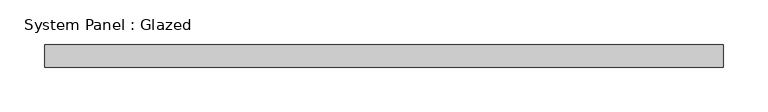
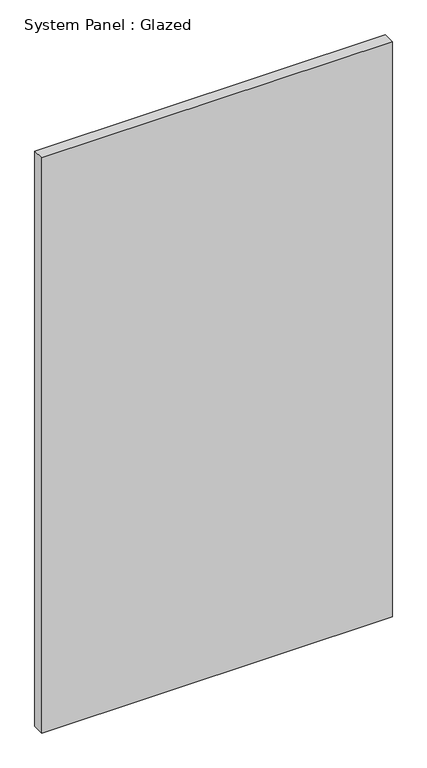
"""IFC4 building model written with IfcOpenShell, lengths in millimetres: plate geometry, System Panel : Glazed."""

from ifc_helpers import new_model, si_unit, origin, origin_with_axes, place, context, project, spatial, polyline, outline, extrude, source, transform, mapped, element, save


def system_panel_glazed_920592d8(model_context):
    return source(origin(), model_context, "Body", "SweptSolid", [
        extrude(outline(polyline([(381.0, 19.05), (-381.0, 19.05), (-381.0, 44.45), (381.0, 44.45), (381.0, 19.05)])), origin_with_axes(), (0.0, 0.0, 1.0), 1320.8),
    ])


if __name__ == "__main__":
    model = new_model("IFC4")
    model_context = context("Model", 3, world=origin())
    ifc_project = project(units=[si_unit("LENGTHUNIT", "METRE", prefix="MILLI")], contexts=[model_context])
    site = spatial("IfcSite", under=ifc_project)
    building = spatial("IfcBuilding", under=site)
    placement = place(None, origin())
    system_panel_glazed_shape = system_panel_glazed_920592d8(model_context)
    element("IfcPlate", 1, ObjectType="System Panel : Glazed", at=placement, inside=building, context=model_context, shape_type="MappedRepresentation", body=[
        mapped(system_panel_glazed_shape, transform((0.0, 0.0, 0.0), x_axis=(1.0, 0.0, 0.0), y_axis=(0.0, 1.0, 0.0), z_axis=(0.0, 0.0, 1.0))),
    ])
    save(model, "model.ifc")

# Revit data of these elements
# Type "System Panel : Glazed"
#   Construction Type Id = "GSP4R"
#   Analytic Construction = "1/8 in Pilkington single glazing"
#   Visual Light Transmittance = 0.9
#   Solar Heat Gain Coefficient = 0.86
#   Heat Transfer Coefficient (U) = 1.18115 BTU/(h·ft²·°F)
# Element 1 (IfcPlate, "System Panel : Glazed")
#   Materials on its faces: "Glass"
# Materials
#   "Glass": class "Glass", colour RGB 0 128 192, transparency 0.75, Description = "Soda Lime Glass", Cost = 0
